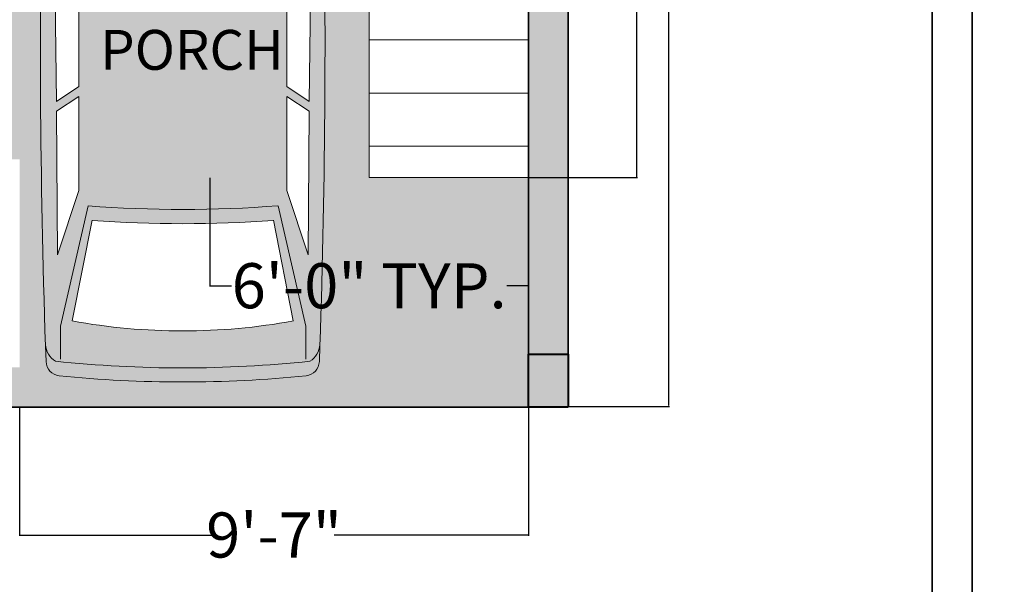
# Model space of a CAD drawing. Units: inches. Extents: x 1077 to 2505, y 1892 to 2728.
# Tile 7 of 26: x 1433 to 1655, y 2048 to 2176. Entities that reach past the tile are written whole.
import ezdxf

# ---------------------------------------------------------------- set-up
doc = ezdxf.new("R2010")
doc.units = ezdxf.units.IN
doc.linetypes.add('ACAD_ISO02W100', pattern=[15, 12, -3])
doc.layers.get('Defpoints').update_dxf_attribs({"color": 220, "linetype": 'ACAD_ISO02W100'})
for name, color, linetype, lineweight in [('A-ANNO-DIMS', 2, 'Continuous', 18), ('A-ANNO-TTLB', 7, 'Continuous', 35), ('A-AREA-IDEN', 7, 'Continuous', 18), ('A-COLS', 7, 'Continuous', 40), ('A-FLOR-STRS', 7, 'Continuous', 18), ('A-FURNITURE', 251, 'Continuous', 5), ('A-SITE-VEHI', 8, 'Continuous', 13), ('A-WALL-PATT', 7, 'Continuous', 9), ('WALL', 7, 'Continuous', 35)]:
    doc.layers.add(name, color=color, linetype=linetype, lineweight=lineweight)
doc.layers.add('A-FLOR-PATT', color=254, linetype='Continuous', lineweight=9, true_color=0xd7ebd2)
doc.styles.get("Standard").update_dxf_attribs({"font": 'arial.ttf'})
doc.dimstyles.get("Standard").update_dxf_attribs({"dimtxt": 10.18, "dimasz": 0.18, "dimexe": 0.18, "dimexo": 0.0625, "dimgap": 0.09, "dimtad": 0, "dimtih": 1, "dimtoh": 1, "dimdec": 0, "dimzin": 0, "dimdsep": 46, "dimlunit": 3, "dimtxsty": 'Standard', "dimcen": 0.09, "dimadec": 0, "dimazin": 0, "dimtfac": 1, "dimtdec": 0, "dimtofl": 0, "dimtmove": 0, "dimatfit": 3, "dimfxl": 1, "dimtolj": 1, "dimtzin": 0, "dimarcsym": 0})

# ---------------------------------------------------------------- blocks, each defined once
blk = doc.blocks.new('CAR')
at = {"layer": 'A-FURNITURE'}
for p, q in [((2677.91, 1665.57), (2683.24, 1629.33)), ((2722.63, 1665.57), (2717.3, 1629.33)), ((2672.85, 1620.44), (2676.61, 1608)), ((2727.48, 1620.44), (2723.73, 1608)), ((2671.15, 1614.07), (2676.73, 1600.01)), ((2671.63, 1575.61), (2671.15, 1614.07)), ((2729.25, 1614.07), (2723.67, 1600.01)), ((2728.77, 1575.61), (2729.25, 1614.07)), ((2676.73, 1600.01), (2676.73, 1578.97)), ((2723.67, 1600.01), (2723.67, 1578.97)), ((2676.73, 1578.97), (2671.63, 1575.61)), ((2723.67, 1578.97), (2728.77, 1575.61)), ((2676.73, 1576.71), (2671.66, 1573.38)), ((2676.73, 1576.71), (2676.73, 1555.46)), ((2723.67, 1576.71), (2723.67, 1555.46)), ((2723.67, 1576.71), (2728.74, 1573.38)), ((2671.9, 1540.91), (2671.66, 1573.38)), ((2728.49, 1540.91), (2728.74, 1573.38)), ((2676.73, 1555.46), (2671.9, 1540.91)), ((2723.67, 1555.46), (2728.49, 1540.91)), ((2678.77, 1552.01), (2672.52, 1524.85)), ((2721.71, 1552.02), (2727.96, 1524.85)), ((2675.22, 1526.01), (2679.74, 1548.74)), ((2725.17, 1526.01), (2720.66, 1548.74)), ((2672.52, 1524.85), (2672.52, 1517.39)), ((2727.96, 1524.85), (2727.96, 1517.39))]:
    blk.add_line(p, q, dxfattribs=at)
for centre, radius, start, end in [((2699.3, 1552.83), 119.14, 76.3976, 102.667), ((2674, 1665.84), 3.34, 104.3452, 166.6607), ((2699.3, 1570.19), 99.28, 73.0347, 105.8141), ((2726.43, 1665.41), 3.34, 13.1156, 74.5941), ((2783.1, 1639.97), 115.47, 166.6607, 186.5655), ((2673.27, 1662.52), 3.34, 107.8179, 168.3942), ((2727.17, 1661.99), 3.34, 11.3249, 70.8826), ((2617.23, 1639.97), 115.47, 353.4345, 13.1156), ((4741.11, 1589.62), 2073.11, 178.89024, 182.01225), ((2700.17, 1579.09), 51.94, 60.0774, 119.9226), ((659.22, 1589.62), 2073.11, 357.98775, 1.10976), ((2675.91, 1621.37), 3.2, 121.1455, 196.7984), ((2724.42, 1621.37), 3.2, 343.2016, 58.8545), ((2679.67, 1608.92), 3.2, 196.7984, 283.6631), ((2700.17, 1519.83), 88.22, 77.0683, 102.9317), ((2720.66, 1608.92), 3.2, 256.3369, 343.2016), ((2700.16, 1829.45), 278.26, 265.5919, 274.4407), ((2700.17, 1827.63), 279.65, 265.7971, 274.2029), ((2700.17, 1663.47), 139.72, 259.6897, 280.3103), ((2674.03, 1521.04), 4.9, 184.3987, 237.5288), ((2726.3, 1521.04), 4.9, 302.4712, 355.6013), ((2672.62, 1516.95), 3.34, 182.1119, 263.4899), ((2700.17, 1791.26), 275.86, 264.0142, 275.9858), ((2727.71, 1516.95), 3.34, 276.5101, 357.8881), ((2700.17, 1790.18), 277.96, 264.2342, 275.7658)]:
    blk.add_arc(centre, radius, start, end, dxfattribs=at)
blk = doc.blocks.new('C1')
h = blk.add_hatch(color=256)
h.dxf.hatch_style = 1
h.paths.add_polyline_path([(1668.56, 2445.41), (1677.56, 2445.41), (1677.56, 2457.41), (1668.56, 2457.41)])
for p, q in [((1668.56, 2457.41), (1677.56, 2457.41)), ((1668.56, 2445.41), (1668.56, 2457.41)), ((1677.56, 2457.41), (1677.56, 2445.41)), ((1677.56, 2445.41), (1668.56, 2445.41))]:
    blk.add_line(p, q)
blk = doc.blocks.new('*D14')
at = {"layer": 'A-ANNO-DIMS', "color": 0, "lineweight": -2, "transparency": 16777216}
for p, q in [((1555.59, 2651.66), (1579.43, 2651.66)), ((1579.25, 2651.48), (1579.25, 2375.3)), ((1579.25, 2088.54), (1579.25, 2364.72)), ((1555.59, 2088.36), (1579.43, 2088.36))]:
    blk.add_line(p, q, dxfattribs=at)
at = {"layer": 'A-ANNO-DIMS', "color": 0, "transparency": 16777216}
for points in [[(1579.22, 2651.48), (1579.28, 2651.48), (1579.25, 2651.66)], [(1579.22, 2088.54), (1579.28, 2088.54), (1579.25, 2088.36)]]:
    blk.add_solid(points, dxfattribs=at)
at = {"layer": 'Defpoints', "color": 0, "transparency": 16777216}
for p in [(1555.53, 2651.66), (1555.53, 2088.36), (1579.25, 2088.36)]:
    blk.add_point(p, dxfattribs=at)
at = {"layer": 'A-ANNO-DIMS', "color": 0, "transparency": 16777216, "insert": (1579.25, 2370.01), "char_height": 10.18, "attachment_point": 5}
blk.add_mtext('\\A1;46\'-11"', dxfattribs=at)
blk = doc.blocks.new('STAIR-PLAN-RETURN')
for p, q in [((0, 163.08), (0, 127.08)), ((12, 163.08), (12, 127.08)), ((24, 163.08), (24, 127.08)), ((36, 163.08), (36, 0)), ((36, 163.08), (36, 127.08)), ((0, 127.08), (72, 127.08)), ((36, 115.08), (72, 115.08)), ((36, 103.08), (72, 103.08)), ((36, 91.08), (72, 91.08)), ((36, 79.08), (72, 79.08)), ((36, 67.08), (72, 67.08)), ((36, 55.08), (72, 55.08)), ((36, 43.08), (72, 43.08)), ((36, 31.08), (72, 31.08)), ((36, 19.08), (72, 19.08)), ((36, 7.08), (72, 7.08)), ((72, 0), (36, 0))]:
    blk.add_line(p, q)
blk = doc.blocks.new('SHEET-FRAME-RESIDENTIAL')
for points in [[(0, 830.04), (543.52, 830.04), (543.52, 0), (0, 0)], [(9, 821.04), (534.52, 821.04), (534.52, 9), (9, 9)]]:
    blk.add_lwpolyline(points, close=True)
blk = doc.blocks.new('*D44')
at = {"layer": 'A-ANNO-DIMS', "color": 0, "lineweight": -2, "transparency": 16777216}
for p, q in [((1547.59, 2303.16), (1572.17, 2303.16)), ((1571.99, 2302.98), (1571.99, 2226.98)), ((1571.99, 2140.26), (1571.99, 2216.26)), ((1547.59, 2140.08), (1572.17, 2140.08))]:
    blk.add_line(p, q, dxfattribs=at)
at = {"layer": 'A-ANNO-DIMS', "color": 0, "transparency": 16777216}
for points in [[(1571.96, 2302.98), (1572.02, 2302.98), (1571.99, 2303.16)], [(1571.96, 2140.26), (1572.02, 2140.26), (1571.99, 2140.08)]]:
    blk.add_solid(points, dxfattribs=at)
at = {"layer": 'Defpoints', "color": 0, "transparency": 16777216}
for p in [(1547.53, 2303.16), (1571.99, 2303.16), (1547.53, 2140.08)]:
    blk.add_point(p, dxfattribs=at)
at = {"layer": 'A-ANNO-DIMS', "color": 0, "transparency": 16777216, "insert": (1571.99, 2221.62), "char_height": 10.18, "attachment_point": 5}
blk.add_mtext('\\A1;RETURN STAIR 13\'-7" TYP.', dxfattribs=at)
blk = doc.blocks.new('*D45')
at = {"layer": 'A-ANNO-DIMS', "color": 0, "lineweight": -2, "transparency": 16777216}
for p, q in [((1475.53, 2140.02), (1475.53, 2115.44)), ((1547.53, 2140.02), (1547.53, 2115.44)), ((1475.71, 2115.62), (1480.38, 2115.62)), ((1547.35, 2115.62), (1542.67, 2115.62))]:
    blk.add_line(p, q, dxfattribs=at)
at = {"layer": 'A-ANNO-DIMS', "color": 0, "transparency": 16777216}
for points in [[(1475.71, 2115.65), (1475.71, 2115.59), (1475.53, 2115.62)], [(1547.35, 2115.65), (1547.35, 2115.59), (1547.53, 2115.62)]]:
    blk.add_solid(points, dxfattribs=at)
at = {"layer": 'Defpoints', "color": 0, "transparency": 16777216}
for p in [(1475.53, 2140.08), (1547.53, 2140.08), (1547.53, 2115.62)]:
    blk.add_point(p, dxfattribs=at)
at = {"layer": 'A-ANNO-DIMS', "color": 0, "transparency": 16777216, "insert": (1511.53, 2115.62), "char_height": 10.18, "attachment_point": 5}
blk.add_mtext('\\A1;6\'-0" TYP.', dxfattribs=at)
blk = doc.blocks.new('*D67')
at = {"layer": 'A-ANNO-DIMS', "color": 0, "lineweight": -2, "transparency": 16777216}
for p, q in [((1432.53, 2088.1), (1432.53, 2059.13)), ((1547.53, 2088.1), (1547.53, 2059.13)), ((1432.71, 2059.31), (1476.41, 2059.31)), ((1547.35, 2059.31), (1503.65, 2059.31))]:
    blk.add_line(p, q, dxfattribs=at)
at = {"layer": 'A-ANNO-DIMS', "color": 0, "transparency": 16777216}
for points in [[(1432.71, 2059.34), (1432.71, 2059.28), (1432.53, 2059.31)], [(1547.35, 2059.34), (1547.35, 2059.28), (1547.53, 2059.31)]]:
    blk.add_solid(points, dxfattribs=at)
at = {"layer": 'Defpoints', "color": 0, "transparency": 16777216}
for p in [(1432.53, 2088.16), (1547.53, 2088.16), (1547.53, 2059.31)]:
    blk.add_point(p, dxfattribs=at)
at = {"layer": 'A-ANNO-DIMS', "color": 0, "transparency": 16777216, "insert": (1490.03, 2059.31), "char_height": 10.18, "attachment_point": 5}
blk.add_mtext('\\A1;9\'-7"', dxfattribs=at)

msp = doc.modelspace()

# ---------------------------------------------------------------- hatches: boundary and pattern name
at = {"layer": 'A-FLOR-PATT', "transparency": 33554559}
h = msp.add_hatch(color=256, dxfattribs=at)
h.dxf.hatch_style = 1
h.paths.add_polyline_path([(1395.53, 2577.16), (1374.83, 2577.16), (1350.83, 2577.19), (1350.83, 2577.16), (1329.53, 2577.16), (1329.53, 2480.16), (1329.53, 2469.16), (1325.53, 2469.16), (1325.53, 2515.13), (1307.53, 2515.13), (1307.53, 2577.16), (1269.31, 2577.16), (1221.31, 2577.15), (1221.31, 2577.16), (1187.53, 2577.16), (1187.53, 2433.16), (1289.53, 2433.16), (1289.53, 2429.16), (1263.53, 2429.16), (1187.53, 2429.16), (1187.53, 2395.02), (1187.53, 2395.02), (1187.53, 2371.02), (1187.53, 2371.02), (1187.53, 2307.16), (1259.53, 2307.16), (1259.53, 2399.16), (1263.53, 2399.16), (1263.53, 2307.16), (1289.53, 2307.16), (1289.53, 2306.23), (1325.53, 2306.23), (1325.53, 2307.16), (1329.53, 2307.16), (1329.53, 2306.23), (1365.53, 2306.23), (1365.53, 2307.16), (1432.53, 2307.16), (1432.53, 2088.16), (1547.53, 2088.16), (1547.53, 2140.08), (1511.53, 2140.08), (1511.53, 2267.16), (1475.53, 2267.16), (1475.53, 2303.16), (1468.53, 2303.16), (1468.53, 2307.16), (1547.53, 2307.16), (1547.53, 2348.22), (1547.53, 2396.22), (1547.53, 2429.16), (1435.53, 2429.16), (1435.53, 2433.16), (1476.35, 2433.16), (1476.35, 2451.18), (1547.53, 2451.18), (1547.53, 2577.16), (1499.53, 2577.16), (1499.53, 2586.16), (1547.53, 2586.16), (1547.53, 2642.16), (1518.18, 2642.16), (1518.18, 2642.05), (1494.15, 2642.05), (1494.15, 2642.16), (1469.53, 2642.16), (1469.53, 2577.16), (1399.53, 2577.16), (1399.53, 2429.16), (1325.53, 2429.16), (1325.53, 2433.16), (1329.53, 2433.16), (1395.53, 2433.16), (1395.53, 2480.16), (1359.53, 2480.16), (1359.53, 2484.16), (1395.53, 2484.16)])
h.paths.add_polyline_path([(1357.65, 2482.07), (1355.65, 2482.07), (1355.65, 2481.07, 0.414214), (1356.65, 2480.07), (1344.65, 2480.07), (1344.65, 2477.06), (1343.27, 2477.06), (1343.27, 2480.07), (1330.65, 2480.07, -0.414214), (1329.65, 2481.07), (1329.65, 2484.07), (1331.65, 2484.07), (1331.65, 2510.07, -0.446908)], flags=16)
h.paths.add_polyline_path([(1305.09, 2559.18), (1288.89, 2559.18), (1288.89, 2575.38), (1305.09, 2575.38)], flags=16)
h.paths.add_polyline_path([(1304.19, 2560.08), (1289.79, 2560.08), (1289.79, 2574.48), (1304.19, 2574.48)], flags=0)
h.paths.add_polyline_path([(1287.99, 2500.68, -0.414214), (1287.09, 2499.78), (1265.14, 2499.78), (1224.09, 2499.78, -0.414214), (1223.19, 2500.68), (1223.19, 2557.16), (1223.19, 2571.74), (1223.19, 2575.38), (1287.99, 2575.38), (1287.99, 2571.74), (1287.09, 2571.74, -0.414214), (1287.99, 2570.84)], flags=16)
h.paths.add_polyline_path([(1292.98, 2569.05, -1), (1300.92, 2569.05, -1)], flags=0)
h.paths.add_polyline_path([(1293.32, 2569.05, -1), (1300.58, 2569.05, -1)], flags=0)
h.paths.add_polyline_path([(1322.8, 2462.21), (1322.8, 2431.71), (1323.05, 2430.71), (1323.05, 2431.71), (1321.8, 2431.71), (1321.8, 2462.19, 0.404641), (1292.3, 2431.71), (1292.05, 2430.71, -0.414214), (1291.55, 2430.21), (1291.05, 2430.21), (1291.05, 2429.71, -0.414214), (1290.55, 2429.21), (1289.55, 2429.21), (1289.55, 2434.21), (1290.55, 2434.21, -0.414214), (1291.05, 2433.71), (1291.05, 2433.21), (1291.55, 2433.21, -0.414214), (1292.05, 2432.71), (1292.3, 2431.71, -0.414214)], flags=16)
h.paths.add_polyline_path([(1287.82, 2548.28, 0.292232), (1279.17, 2536.8, 0.052719), (1223.93, 2548.28), (1223.28, 2548.28), (1223.28, 2557.16), (1223.93, 2557.16), (1245.42, 2557.16, -0.117785), (1245.77, 2557.93, -0.059418), (1254.87, 2567.02, -0.379859), (1257.28, 2566.88, -0.02509), (1261.41, 2563.32, -0.025935), (1265.65, 2567.02, -0.379859), (1268.06, 2566.88, -0.061767), (1277.52, 2557.43, -0.069393), (1277.82, 2557.16), (1287.82, 2557.16)], flags=0)
h.paths.add_polyline_path([(1263.47, 2548.28), (1260.56, 2548.28, -0.015371), (1258.01, 2546.13, -0.429576), (1255.37, 2546.06, -0.016036), (1252.69, 2548.28), (1223.28, 2548.28), (1223.28, 2554.42), (1246.78, 2554.42, 0.055344), (1255.37, 2546.06, 0.331768), (1257.52, 2545.74, 0.027343), (1262, 2549.64, 0.00919)], flags=0)
h.paths.add_polyline_path([(1295.56, 2568.34), (1296.87, 2569.09), (1296.87, 2570.6, 0.399698), (1295.39, 2569.05, 0.119004)], flags=0)
h.paths.add_polyline_path([(1295.21, 2569.05, -1), (1298.68, 2569.05, -1)], flags=0)
h.paths.add_polyline_path([(1296.95, 2568.96), (1297.03, 2569), (1297.03, 2569.09), (1296.99, 2569.11), (1296.91, 2568.98)], flags=0)
h.paths.add_polyline_path([(1402.28, 2462.19, -0.414214), (1432.78, 2431.69), (1433.03, 2432.69), (1432.78, 2431.69, 0.404641), (1403.28, 2462.17), (1403.28, 2431.69), (1402.03, 2431.69), (1402.03, 2430.69, -0.414214), (1401.53, 2430.19), (1401.03, 2430.19), (1401.03, 2429.69, -0.414214), (1400.53, 2429.19), (1399.53, 2429.19), (1399.53, 2434.19), (1400.53, 2434.19, -0.414214), (1401.03, 2433.69), (1401.03, 2433.19), (1401.53, 2433.19, -0.414214), (1402.03, 2432.69)], flags=16)
h.paths.add_polyline_path([(1470.16, 2535.21, -0.414214), (1471.06, 2536.11), (1527.54, 2536.11), (1542.12, 2536.11), (1545.76, 2536.11), (1545.76, 2471.31), (1542.12, 2471.31), (1542.12, 2472.21, -0.414214), (1541.22, 2471.31), (1471.06, 2471.31, -0.414214), (1470.16, 2472.21), (1470.16, 2494.16)], flags=16)
h.paths.add_polyline_path([(1483.07, 2536.11, 0.253465), (1480.11, 2526.15, 0.2538), (1470.15, 2523.19)], flags=16)
h.paths.add_polyline_path([(1223.19, 2512.69, 0.253465), (1233.14, 2509.74, 0.2538), (1236.1, 2499.77)], flags=16)
h.paths.add_polyline_path([(1469.77, 2578.72), (1469.77, 2581.72), (1471.77, 2581.72), (1471.77, 2607.72, -0.01951), (1473.77, 2607.68), (1473.77, 2579.72), (1473.77, 2578.72, -0.414214), (1472.77, 2577.72), (1470.77, 2577.72, -0.414214)], flags=16)
h.paths.add_polyline_path([(1382.46, 2398.13), (1395.04, 2398.13), (1395.04, 2399.74), (1382.46, 2399.74)], flags=16)
h.paths.add_polyline_path([(1379.94, 2397.18), (1379.94, 2389.82), (1380.5, 2389.82), (1380.5, 2396.05, -0.41429), (1381.06, 2396.61), (1396.47, 2396.61, -0.414213), (1397.03, 2396.05), (1397.03, 2389.82), (1397.59, 2389.82), (1397.59, 2397.18)], flags=16)
h.paths.add_polyline_path([(1263.37, 2428.14), (1263.37, 2426.14, -0.414214), (1262.37, 2425.14), (1261.37, 2425.14), (1233.41, 2425.14, 0.400854), (1259.37, 2401.04), (1259.37, 2401.14), (1261.37, 2401.14, -0.446908), (1233.37, 2427.14), (1259.37, 2427.14), (1259.37, 2429.14), (1262.37, 2429.14, -0.414214)], flags=16)
h.paths.add_polyline_path([(1404.79, 2398.13), (1417.37, 2398.13), (1417.37, 2399.74), (1404.79, 2399.74)], flags=16)
h.paths.add_polyline_path([(1402.27, 2397.18), (1404.79, 2398.13), (1417.37, 2398.13), (1419.92, 2397.18)], flags=16)
h.paths.add_polyline_path([(1432.26, 2383.16), (1432.26, 2370.59), (1433.87, 2370.59), (1433.87, 2383.16)], flags=16)
h.paths.add_polyline_path([(1431.3, 2385.69), (1423.84, 2385.69), (1423.84, 2385.13), (1430.18, 2385.13, -0.41429), (1430.74, 2384.57), (1430.74, 2369.16, -0.414237), (1430.18, 2368.6), (1423.84, 2368.6), (1423.84, 2368.03), (1431.3, 2368.03)], flags=16)
h.paths.add_polyline_path([(1417.37, 2351.16), (1417.37, 2349.54), (1418.9, 2349.54, 0.414236), (1419.92, 2350.56), (1419.92, 2352.11)], flags=16)
h.paths.add_polyline_path([(1395.04, 2351.16), (1395.04, 2349.54), (1396.58, 2349.54, 0.414235), (1397.59, 2350.56), (1397.59, 2352.11)], flags=16)
h.paths.add_polyline_path([(1366.7, 2370.05), (1365.09, 2370.05), (1365.09, 2368.52, 0.414235), (1366.11, 2367.5), (1367.66, 2367.5)], flags=16)
h.paths.add_polyline_path([(1419.36, 2359.47), (1419.36, 2353.24, -0.41419), (1418.8, 2352.68), (1403.39, 2352.68, -0.414137), (1402.83, 2353.24), (1402.83, 2359.47), (1397.03, 2359.47), (1397.03, 2353.24, -0.414189), (1396.47, 2352.68), (1381.06, 2352.68, -0.414137), (1380.5, 2353.24), (1380.5, 2359.47)], flags=16)
h.paths.add_polyline_path([(1222.29, 2559.18), (1206.09, 2559.18), (1206.09, 2575.38), (1222.29, 2575.38)], flags=16)
h.paths.add_polyline_path([(1221.39, 2560.08), (1206.99, 2560.08), (1206.99, 2574.48), (1221.39, 2574.48)], flags=0)
h.paths.add_polyline_path([(1482, 2577.72), (1482, 2580.73), (1483.38, 2580.73), (1483.38, 2577.72), (1484.77, 2577.72), (1484.77, 2574.72), (1483.38, 2574.72), (1483.38, 2577.72)], flags=16)
h.paths.add_polyline_path([(1266.37, 2415.53), (1266.37, 2414.14), (1263.37, 2414.14), (1263.37, 2415.53), (1260.36, 2415.53), (1260.36, 2416.91), (1263.37, 2416.91), (1263.37, 2415.53)], flags=16)
h.paths.add_polyline_path([(1210.26, 2569.05, -1), (1218.19, 2569.05, -1)], flags=0)
h.paths.add_polyline_path([(1210.6, 2569.05, -1), (1217.85, 2569.05, -1)], flags=0)
h.paths.add_polyline_path([(1212.84, 2568.34), (1214.15, 2569.09), (1214.15, 2570.6, 0.399698), (1212.67, 2569.05, 0.119004)], flags=0)
h.paths.add_polyline_path([(1212.49, 2569.05, -1), (1215.96, 2569.05, -1)], flags=0)
h.paths.add_polyline_path([(1214.23, 2568.96), (1214.3, 2568.91), (1214.3, 2569)], flags=0)
h.paths.add_polyline_path([(1507.18, 2480.12, 0.052719), (1518.66, 2535.36), (1518.66, 2536.01), (1527.54, 2536.01), (1527.54, 2535.36), (1527.54, 2513.88, -0.117785), (1528.31, 2513.53, -0.059418), (1537.4, 2504.43, -0.379859), (1537.26, 2502.01, -0.02509), (1533.7, 2497.89, -0.025935), (1537.4, 2493.64, -0.379859), (1537.26, 2491.23, -0.061767), (1527.8, 2481.77, -0.069393), (1527.54, 2481.47), (1527.54, 2471.47), (1518.66, 2471.47, 0.292232)], flags=0)
h.paths.add_polyline_path([(1516.43, 2503.92, -0.016036), (1518.66, 2506.6), (1518.66, 2536.01), (1524.8, 2536.01), (1524.8, 2512.51, 0.055344), (1516.43, 2503.92, 0.331768), (1516.12, 2501.77, 0.027343), (1520.01, 2497.29, 0.00919), (1518.66, 2495.82), (1518.66, 2498.73, -0.015371), (1516.5, 2501.28, -0.429576)], flags=0)
h.paths.add_polyline_path([(1499.63, 2625.5, -0.171636), (1502.82, 2631.01), (1502.82, 2633.37), (1498.68, 2633.37, -0.414214), (1497.7, 2634.36), (1497.7, 2640.66, -0.414214), (1498.68, 2641.64), (1514.82, 2641.64, -0.414214), (1515.81, 2640.66), (1515.81, 2634.36, -0.414214), (1514.82, 2633.37), (1510.69, 2633.37), (1510.69, 2631.01, -0.171636), (1513.88, 2625.5, -0.258205), (1509.31, 2614.47), (1504.19, 2614.47, -0.258205)], flags=16)
h.paths.add_polyline_path([(1501.2, 2625.5, -0.171636), (1504.39, 2631.01), (1509.12, 2631.01, -0.171636), (1512.3, 2625.5, -0.210384), (1509.35, 2616.02), (1504.16, 2616.02, -0.210384)], flags=0)
h.paths.add_polyline_path([(1529.56, 2537.01), (1529.56, 2553.21), (1545.76, 2553.21), (1545.76, 2537.01)], flags=16)
h.paths.add_polyline_path([(1530.46, 2537.91), (1530.46, 2552.31), (1544.86, 2552.31), (1544.86, 2537.91)], flags=0)
h.paths.add_polyline_path([(1535.45, 2545.07, -1), (1543.39, 2545.07, -1)], flags=0)
h.paths.add_polyline_path([(1535.8, 2545.07, -1), (1543.05, 2545.07, -1)], flags=0)
h.paths.add_polyline_path([(1529.56, 2470.41), (1545.76, 2470.41), (1545.76, 2454.21), (1529.56, 2454.21)], flags=16)
h.paths.add_polyline_path([(1541.16, 2544.99), (1540.98, 2544.99, -0.544606), (1538.71, 2543.68), (1538.62, 2543.53, 0.547962)], flags=0)
h.paths.add_polyline_path([(1530.46, 2469.51), (1544.86, 2469.51), (1544.86, 2455.11), (1530.46, 2455.11)], flags=0)
h.paths.add_polyline_path([(1539.47, 2545.14), (1539.42, 2545.22), (1539.38, 2545.14)], flags=0)
h.paths.add_polyline_path([(1543.39, 2462.34, -1), (1535.45, 2462.34, -1)], flags=0)
h.paths.add_polyline_path([(1543.05, 2462.34, -1), (1535.8, 2462.34, -1)], flags=0)
h.paths.add_polyline_path([(1541.16, 2462.27), (1540.98, 2462.27, -0.544606), (1538.71, 2460.96), (1538.62, 2460.8, 0.547962)], flags=0)
h.paths.add_polyline_path([(1539.47, 2462.42), (1539.42, 2462.5), (1539.38, 2462.42)], flags=0)
h.paths.add_polyline_path([(1435.32, 2335.25, -0.414214), (1465.82, 2304.75), (1466.07, 2305.75), (1465.82, 2304.75, 0.404641), (1436.32, 2335.23), (1436.32, 2304.75), (1435.07, 2304.75), (1435.07, 2303.75, -0.414214), (1434.57, 2303.25), (1434.07, 2303.25), (1434.07, 2302.75, -0.414214), (1433.57, 2302.25), (1432.57, 2302.25), (1432.57, 2307.25), (1433.57, 2307.25, -0.414214), (1434.07, 2306.75), (1434.07, 2306.25), (1434.57, 2306.25, -0.414214), (1435.07, 2305.75)], flags=16)
h.paths.add_polyline_path([(1532.13, 2635.71), (1535.43, 2635.71), (1535.43, 2635.89), (1532.13, 2635.89)], flags=16)
edge = h.paths.add_edge_path(flags=16)
edge.add_arc((1535.98, 2632.67), 0.183, 270, 360)
edge.add_line((1536.17, 2632.67), (1536.17, 2639.82))
edge.add_line((1536.17, 2639.82), (1538.29, 2639.82))
edge.add_line((1538.29, 2639.82), (1538.29, 2641.82))
edge.add_line((1538.29, 2641.82), (1533.25, 2641.82))
edge.add_line((1533.25, 2641.82), (1533.25, 2639.82))
edge.add_line((1533.25, 2639.82), (1534.87, 2639.82))
edge.add_line((1534.87, 2639.82), (1534.87, 2639))
edge.add_line((1534.87, 2639), (1533.7, 2639))
edge.add_line((1533.7, 2639), (1533.7, 2639.82))
edge.add_line((1533.7, 2639.82), (1533.25, 2639.82))
edge.add_line((1533.25, 2639.82), (1533.25, 2641.82))
edge.add_line((1533.25, 2641.82), (1538.29, 2641.82))
edge.add_line((1538.29, 2641.82), (1538.29, 2641.34))
edge.add_line((1538.29, 2641.34), (1540.64, 2641.58))
edge.add_line((1540.64, 2641.58), (1540.64, 2641.82))
edge.add_line((1540.64, 2641.82), (1541.5, 2641.82))
edge.add_line((1541.5, 2641.82), (1541.5, 2641.25))
edge.add_line((1541.5, 2641.25), (1541.31, 2639.79))
edge.add_ellipse((1541.09, 2638.95), major_axis=(-1.08, 0), ratio=0.790849, start_angle=180, end_angle=255.2976, ccw=False)
edge.add_line((1542.17, 2638.95), (1542.17, 2638.38))
edge.add_ellipse((1541.09, 2638.38), major_axis=(-1.08, 0), ratio=0.790849, start_angle=0, end_angle=180, ccw=False)
edge.add_line((1540, 2638.38), (1540.01, 2638.87))
edge.add_ellipse((1541.09, 2638.95), major_axis=(-1.08, 0), ratio=0.790849, start_angle=284.7024, end_angle=364.0401, ccw=False)
edge.add_line((1540.78, 2639.75), (1540.78, 2641.25))
edge.add_line((1540.78, 2641.25), (1540.64, 2641.25))
edge.add_line((1540.64, 2641.25), (1538.29, 2641.01))
edge.add_line((1538.29, 2641.01), (1538.29, 2639.82))
edge.add_line((1538.29, 2639.82), (1536.17, 2639.82))
edge.add_line((1536.17, 2639.82), (1536.17, 2632.48))
edge.add_line((1536.17, 2632.48), (1535.98, 2632.48))
h.paths.add_polyline_path([(1496.32, 2250.34, -0.292371), (1498.9, 2247.83, -0.085148), (1501.21, 2208.85, -0.01331), (1500.27, 2098.5, -0.379287), (1497.22, 2095.28, -0.0502), (1441.54, 2095.28, -0.379287), (1438.5, 2098.5, -0.01331), (1437.56, 2208.85, -0.086132), (1439.96, 2248.26, -0.295116), (1442.59, 2250.78, -0.114238)], flags=16)
h.paths.add_polyline_path([(1495.16, 2205.84, -0.355389), (1496.7, 2202.1), (1492.94, 2189.65, -0.398275), (1489.12, 2187.47, 0.113332), (1449.64, 2187.47, -0.398275), (1445.82, 2189.65), (1442.06, 2202.1, -0.355394), (1443.6, 2205.84, -0.265725)], flags=0)
h.paths.add_polyline_path([(1440.37, 2195.72), (1445.94, 2181.67), (1445.94, 2160.63), (1440.84, 2157.26)], flags=0)
h.paths.add_polyline_path([(1498.46, 2195.72), (1497.99, 2157.26), (1492.88, 2160.63), (1492.88, 2181.67)], flags=0)
h.paths.add_polyline_path([(1445.94, 2158.37), (1445.94, 2137.12), (1441.12, 2122.56), (1440.87, 2155.03)], flags=0)
h.paths.add_polyline_path([(1492.88, 2158.37), (1497.96, 2155.03), (1497.71, 2122.56), (1492.88, 2137.12)], flags=0)
h.paths.add_polyline_path([(1489.88, 2130.4), (1494.39, 2107.67, -0.090102), (1444.44, 2107.65), (1448.95, 2130.39, 0.036636)], flags=0)
h.paths.add_polyline_path([(1447.54, 2159.34), (1497.44, 2159.34), (1497.44, 2177.89), (1447.54, 2177.89)], flags=8)
h.paths.add_polyline_path([(1196.44, 2354.84), (1246.65, 2354.84), (1246.65, 2388.43), (1196.44, 2388.43)], flags=24)
h.paths.add_polyline_path([(1296.09, 2360.25), (1353.81, 2360.25), (1353.81, 2393.84), (1296.09, 2393.84)], flags=24)
h.paths.add_polyline_path([(1400.72, 2471.85), (1470.63, 2471.85), (1470.63, 2505.44), (1400.72, 2505.44)], flags=24)
h.paths.add_polyline_path([(1324.78, 2448.48), (1394.95, 2448.48), (1394.95, 2467.02), (1324.78, 2467.02)], flags=24)
h.paths.add_polyline_path([(1335.08, 2531.43), (1389.67, 2531.43), (1389.67, 2565.02), (1335.08, 2565.02)], flags=24)
h.paths.add_polyline_path([(1225.76, 2460), (1295.67, 2460), (1295.67, 2493.58), (1225.76, 2493.58)], flags=24)
h = msp.add_hatch(color=256, dxfattribs=at)
h.dxf.hatch_style = 1
h.paths.add_polyline_path([(1547.53, 2348.22), (1547.53, 2396.22), (1547.53, 2425.11), (1547.53, 2425.11), (1547.53, 2429.16), (1435.53, 2429.16), (1434.03, 2429.21), (1434.03, 2430.19), (1433.03, 2430.19), (1432.78, 2431.69, 0.404641), (1403.28, 2462.17), (1403.28, 2431.69), (1402.03, 2431.69), (1402.03, 2430.19), (1401.03, 2430.19), (1401.03, 2429.19), (1399.53, 2429.19), (1399.53, 2429.19), (1399.53, 2429.16), (1334.67, 2429.16), (1334.67, 2423.95), (1325.67, 2423.95), (1325.67, 2429.16), (1325.53, 2429.16), (1324.05, 2429.24), (1324.05, 2430.21), (1323.05, 2430.21), (1323.05, 2431.71), (1321.8, 2431.71), (1321.8, 2462.19, 0.416544), (1292.05, 2430.73, -0.423614), (1291.55, 2430.21), (1291.05, 2430.21), (1291.05, 2429.21), (1289.55, 2429.21), (1289.53, 2429.21), (1289.53, 2429.16), (1263.37, 2429.16), (1263.37, 2415.53), (1266.37, 2415.53), (1266.37, 2414.14), (1263.37, 2414.14), (1263.37, 2399.16), (1263.53, 2399.16), (1263.53, 2307.16), (1289.53, 2307.16), (1289.53, 2306.23), (1323.26, 2306.23), (1323.26, 2307.21), (1332.26, 2307.21), (1365.53, 2306.23), (1365.53, 2307.16), (1432.53, 2307.16), (1432.57, 2307.16), (1432.57, 2307.25), (1434.07, 2307.25), (1434.07, 2306.25), (1435.32, 2306.25), (1435.32, 2335.25, -0.407346), (1466.07, 2305.73, -0.423614), (1466.57, 2306.25), (1467.07, 2306.25), (1467.07, 2307.25), (1468.57, 2307.25), (1547.53, 2307.16), (1547.53, 2307.2)])
h.paths.add_polyline_path([(1430.74, 2369.16), (1430.74, 2384.57, 0.41429), (1430.18, 2385.13), (1423.84, 2385.13), (1423.84, 2368.6), (1430.18, 2368.6, 0.414237)], flags=16)
h.paths.add_polyline_path([(1432.26, 2383.16), (1432.26, 2370.59), (1433.87, 2370.59), (1433.87, 2383.16)], flags=16)
h.paths.add_polyline_path([(1431.3, 2368.03), (1431.3, 2385.69), (1432.26, 2383.16), (1432.26, 2370.59)], flags=16)
h.paths.add_polyline_path([(1417.37, 2351.16), (1417.37, 2349.54), (1418.9, 2349.54, 0.414236), (1419.92, 2350.56), (1419.92, 2352.11)], flags=16)
h.paths.add_polyline_path([(1403.39, 2352.68), (1418.78, 2352.68, 0.42427), (1419.36, 2353.24), (1419.36, 2359.47), (1402.83, 2359.47), (1402.83, 2353.24, 0.414137)], flags=16)
h.paths.add_polyline_path([(1366.7, 2370.05), (1365.09, 2370.05), (1365.09, 2368.52, 0.414235), (1366.11, 2367.5), (1367.66, 2367.5)], flags=16)
h.paths.add_polyline_path([(1382.46, 2398.13), (1395.04, 2398.13), (1395.04, 2399.74), (1382.46, 2399.74)], flags=16)
h.paths.add_polyline_path([(1396.47, 2396.61), (1381.06, 2396.61, 0.41429), (1380.5, 2396.05), (1380.5, 2389.82), (1397.03, 2389.82), (1397.03, 2396.05, 0.414213)], flags=16)
h.paths.add_polyline_path([(1402.27, 2397.18), (1402.83, 2396.05, -0.414213), (1403.39, 2396.61)], flags=16)
h.paths.add_polyline_path([(1418.8, 2396.61), (1419.36, 2396.61), (1419.36, 2396.05, 0.414237)], flags=16)
h.paths.add_polyline_path([(1404.79, 2398.13), (1417.37, 2398.13), (1417.37, 2399.74), (1404.79, 2399.74)], flags=16)
h.paths.add_polyline_path([(1381.06, 2352.68, -0.414213), (1380.5, 2353.24), (1380.27, 2352.11)], flags=16)
h.paths.add_polyline_path([(1396.58, 2349.54), (1396.58, 2349.54), (1395.04, 2349.54), (1395.04, 2349.54), (1382.46, 2349.54), (1382.46, 2351.16), (1395.04, 2351.16), (1397.59, 2352.11), (1397.59, 2350.56, -0.414235)], flags=16)
h.paths.add_polyline_path([(1379.94, 2397.18), (1382.46, 2398.13), (1395.04, 2398.13), (1397.59, 2397.18)], flags=16)
h.paths.add_polyline_path([(1368.78, 2384.59, 0.414213), (1368.22, 2384.03), (1367.66, 2367.5), (1367.66, 2385.15)], flags=16)
h.paths.add_polyline_path([(1547.53, 2574.38), (1547.51, 2574.38), (1547.51, 2577.16), (1499.53, 2577.16), (1484.77, 2577.44), (1484.77, 2574.72), (1483.38, 2574.72), (1483.38, 2577.72), (1482, 2577.72), (1469.53, 2577.72), (1469.53, 2577.16), (1401.95, 2577.16), (1401.95, 2574.12), (1399.53, 2574.12), (1399.53, 2434.19), (1401.03, 2434.19), (1401.03, 2433.19), (1402.28, 2433.19), (1402.28, 2462.19, -0.407346), (1433.03, 2432.67, -0.423614), (1433.53, 2433.19), (1434.03, 2433.19), (1434.03, 2434.19), (1435.53, 2434.19), (1476.35, 2433.81), (1476.35, 2451.18), (1547.53, 2451.18)])
h.paths.add_polyline_path([(1470.16, 2535.21, -0.414214), (1471.06, 2536.11), (1527.54, 2536.11), (1542.12, 2536.11), (1545.76, 2536.11), (1545.76, 2471.31), (1542.12, 2471.31), (1542.12, 2472.21, -0.414214), (1541.22, 2471.31), (1471.06, 2471.31, -0.414214), (1470.16, 2472.21), (1470.16, 2494.16)], flags=16)
h.paths.add_polyline_path([(1483.07, 2536.11, 0.253465), (1480.11, 2526.15, 0.2538), (1470.15, 2523.19)], flags=16)
h.paths.add_polyline_path([(1525.55, 2481.52, -0.000893), (1524.8, 2482.24), (1524.8, 2471.47), (1527.54, 2471.47), (1527.54, 2472.12), (1527.54, 2481.47, -0.388819)], flags=0)
h.paths.add_polyline_path([(1518.66, 2536.01), (1527.54, 2536.01), (1527.54, 2535.36), (1527.54, 2513.88, -0.117785), (1528.31, 2513.53, -0.059418), (1537.4, 2504.43, -0.379859), (1537.26, 2502.01, -0.02509), (1533.7, 2497.89, 0.033431), (1528.3, 2502.74, 0.308459), (1526.25, 2502.88, 0.047827), (1518.66, 2495.82), (1518.66, 2498.73, -0.015371), (1516.5, 2501.28, -0.429576), (1516.43, 2503.92, -0.016036), (1518.66, 2506.6)], flags=0)
h.paths.add_polyline_path([(1529.56, 2537.01), (1529.56, 2553.21), (1545.76, 2553.21), (1545.76, 2537.01)], flags=16)
h.paths.add_polyline_path([(1530.46, 2537.91), (1530.46, 2552.31), (1544.86, 2552.31), (1544.86, 2537.91)], flags=0)
h.paths.add_polyline_path([(1535.8, 2545.07, -1), (1543.05, 2545.07, -1)], flags=0)
h.paths.add_polyline_path([(1541.16, 2544.99), (1540.98, 2544.99, -0.544606), (1538.71, 2543.68), (1538.62, 2543.53, 0.547962)], flags=0)
h.paths.add_polyline_path([(1539.47, 2545.14), (1539.42, 2545.22), (1539.38, 2545.14)], flags=0)
h.paths.add_polyline_path([(1529.56, 2470.41), (1545.76, 2470.41), (1545.76, 2454.21), (1529.56, 2454.21)], flags=16)
h.paths.add_polyline_path([(1530.46, 2469.51), (1544.86, 2469.51), (1544.86, 2455.11), (1530.46, 2455.11)], flags=0)
h.paths.add_polyline_path([(1535.8, 2462.34, -1), (1543.05, 2462.34, -1)], flags=0)
h.paths.add_polyline_path([(1541.16, 2462.27), (1540.98, 2462.27, -0.544606), (1538.71, 2460.96), (1538.62, 2460.8, 0.547962)], flags=0)
h.paths.add_polyline_path([(1539.47, 2462.42), (1539.42, 2462.5), (1539.38, 2462.42)], flags=0)
h.paths.add_polyline_path([(1395.53, 2574.12), (1392.95, 2574.12), (1392.95, 2577.16), (1374.83, 2577.16), (1350.83, 2577.19), (1350.83, 2577.16), (1332.07, 2577.16), (1332.07, 2574), (1329.53, 2574), (1329.53, 2484.07), (1331.65, 2484.07), (1331.65, 2510.07, -0.423677), (1357.76, 2484.07), (1359.53, 2484.07), (1359.53, 2484.16), (1395.53, 2484.16)], flags=17)
h.paths.add_polyline_path([(1395.53, 2480.16), (1359.06, 2480.16, 0.437533), (1359.53, 2481.55), (1359.53, 2484.16), (1395.53, 2484.16), (1395.53, 2574.12), (1392.95, 2574.12), (1392.95, 2577.16), (1374.83, 2577.16), (1350.83, 2577.19), (1350.83, 2577.16), (1332.07, 2577.16), (1332.07, 2574), (1329.53, 2574), (1329.53, 2484.07), (1329.65, 2484.07), (1329.65, 2481.07), (1329.53, 2480.16), (1329.53, 2469.16), (1325.53, 2469.16), (1325.53, 2515.13), (1307.53, 2515.13), (1307.53, 2577.16), (1269.31, 2577.16), (1221.31, 2577.15), (1221.31, 2577.16), (1187.61, 2577.16), (1187.61, 2574.03), (1187.53, 2433.16), (1289.55, 2433.16), (1289.55, 2434.21), (1291.05, 2434.21), (1291.05, 2433.21), (1292.05, 2433.21), (1292.3, 2431.71, -0.414214), (1322.8, 2462.21), (1323.05, 2432.71, -0.414214), (1323.55, 2433.21), (1324.05, 2433.21), (1324.05, 2434.21), (1325.67, 2434.21), (1325.67, 2435.95), (1334.67, 2435.95), (1334.67, 2433.16), (1395.53, 2433.16)])
h.paths.add_polyline_path([(1344.65, 2480.07), (1344.65, 2477.06), (1343.27, 2477.06), (1343.27, 2480.07), (1332.65, 2480.07, 0.414214), (1333.65, 2481.07), (1333.65, 2482.07), (1331.65, 2482.07), (1331.65, 2484.07), (1331.65, 2510.07, -0.446908), (1357.65, 2482.07), (1355.65, 2482.07), (1355.65, 2481.07, 0.414214), (1356.65, 2480.07)], flags=16)
h.paths.add_polyline_path([(1287.99, 2500.68, -0.414214), (1287.09, 2499.78), (1265.14, 2499.78), (1224.09, 2499.78, -0.414214), (1223.19, 2500.68), (1223.19, 2557.16), (1223.19, 2571.74), (1223.19, 2575.38), (1287.99, 2575.38), (1287.99, 2571.74), (1287.09, 2571.74, -0.414214), (1287.99, 2570.84)], flags=16)
h.paths.add_polyline_path([(1277.77, 2555.17, -0.000893), (1277.05, 2554.42), (1287.82, 2554.42), (1287.82, 2557.16), (1287.17, 2557.16), (1277.82, 2557.16, -0.388819)], flags=0)
h.paths.add_polyline_path([(1223.28, 2548.28), (1223.28, 2557.16), (1223.93, 2557.16), (1245.42, 2557.16, -0.117785), (1245.77, 2557.93, -0.059418), (1254.87, 2567.02, -0.379859), (1257.28, 2566.88, -0.02509), (1261.41, 2563.32, 0.033431), (1256.55, 2557.93, 0.308459), (1256.41, 2555.88, 0.047827), (1263.47, 2548.28), (1260.56, 2548.28, -0.015371), (1258.01, 2546.13, -0.429576), (1255.37, 2546.06, -0.016036), (1252.69, 2548.28)], flags=0)
h.paths.add_polyline_path([(1305.09, 2559.18), (1288.89, 2559.18), (1288.89, 2575.38), (1305.09, 2575.38)], flags=16)
h.paths.add_polyline_path([(1304.19, 2560.08), (1289.79, 2560.08), (1289.79, 2574.48), (1304.19, 2574.48)], flags=0)
h.paths.add_polyline_path([(1300.58, 2569.05, -1), (1293.32, 2569.05, -1)], flags=0)
h.paths.add_polyline_path([(1223.19, 2512.69, 0.253465), (1233.14, 2509.74, 0.2538), (1236.1, 2499.77)], flags=16)
h.paths.add_polyline_path([(1295.56, 2568.34), (1296.87, 2569.09), (1296.87, 2570.6, 0.399698), (1295.39, 2569.05, 0.119004)], flags=0)
h.paths.add_polyline_path([(1295.21, 2569.05, -1), (1298.68, 2569.05, -1)], flags=0)
h.paths.add_polyline_path([(1296.95, 2568.96), (1297.03, 2569), (1297.03, 2569.09), (1296.99, 2569.11), (1296.91, 2568.98)], flags=0)
h.paths.add_polyline_path([(1222.29, 2559.18), (1206.09, 2559.18), (1206.09, 2575.38), (1222.29, 2575.38)], flags=16)
h.paths.add_polyline_path([(1221.39, 2560.08), (1206.99, 2560.08), (1206.99, 2574.48), (1221.39, 2574.48)], flags=0)
h.paths.add_polyline_path([(1217.85, 2569.05, -1), (1210.6, 2569.05, -1)], flags=0)
h.paths.add_polyline_path([(1212.84, 2568.34), (1214.15, 2569.09), (1214.15, 2570.6, 0.399698), (1212.67, 2569.05, 0.119004)], flags=0)
h.paths.add_polyline_path([(1212.49, 2569.05, -1), (1215.96, 2569.05, -1)], flags=0)
h.paths.add_polyline_path([(1214.23, 2568.96), (1214.3, 2569), (1214.3, 2569.09), (1214.26, 2569.11), (1214.19, 2568.98)], flags=0)
h.paths.add_polyline_path([(1259.53, 2399.14), (1259.37, 2399.14), (1259.37, 2401.04, -0.423677), (1233.37, 2427.14), (1259.37, 2427.14), (1259.37, 2429.16), (1187.53, 2429.16), (1187.53, 2395.02), (1187.53, 2395.02), (1187.53, 2371.02), (1187.53, 2371.02), (1187.53, 2311.49), (1187.55, 2311.49), (1187.55, 2307.16), (1259.53, 2307.16)])
h.paths.add_polyline_path([(1323.26, 2295.21), (1323.26, 2304.23), (1289.53, 2304.23), (1289.53, 2303.16), (1187.55, 2303.16), (1187.55, 2299.49), (1178.53, 2299.49), (1178.53, 2267.66), (1178.53, 2219.66), (1182.03, 2219.66), (1182.03, 2267.67), (1184.03, 2267.67), (1184.03, 2219.66), (1187.53, 2219.66), (1187.53, 2153.16), (1228.13, 2153.16), (1276.13, 2153.16), (1276.13, 2153.16), (1324.54, 2153.16), (1324.54, 2154.67), (1325.54, 2154.67), (1325.54, 2155.92), (1296.54, 2155.92, -0.407346), (1326.06, 2186.67, -0.423614), (1325.54, 2187.17), (1325.54, 2187.67), (1324.54, 2187.67), (1324.54, 2189.17), (1325.43, 2295.21)])
h.paths.add_polyline_path([(1432.53, 2307.16), (1365.53, 2307.16), (1365.53, 2306.23), (1365.53, 2303.16), (1428.53, 2303.16), (1428.53, 2221.2), (1428.57, 2221.2), (1428.57, 2197.2), (1428.53, 2197.16), (1428.53, 2303.01), (1404.46, 2303.01), (1404.46, 2221.2), (1329.53, 2221.2), (1329.53, 2307.16), (1325.53, 2307.16), (1325.53, 2295.21), (1325.43, 2295.21), (1324.54, 2189.17), (1324.54, 2187.67), (1326.04, 2187.67, 1.016365), (1326.06, 2186.67, 0.407348), (1296.54, 2155.92), (1325.54, 2155.92), (1325.54, 2154.67), (1324.54, 2154.67), (1324.54, 2153.16), (1329.53, 2153.16), (1329.53, 2144.16), (1432.53, 2144.16)])
h.paths.add_polyline_path([(1361.95, 2194.26), (1361.95, 2193.16), (1329.53, 2193.16), (1329.53, 2189.16), (1329.54, 2188.17), (1329.54, 2189.16), (1329.53, 2189.16), (1329.53, 2193.16), (1361.95, 2193.16), (1361.95, 2196.26), (1409.95, 2196.26), (1409.95, 2194.26)], flags=16)
h.paths.add_polyline_path([(1377.02, 2200.5), (1345.91, 2200.5), (1345.91, 2218.4), (1347.87, 2218.4), (1347.87, 2219.18), (1374.75, 2219.18), (1374.75, 2218.4), (1377.02, 2218.4)], flags=16)
h.paths.add_polyline_path([(1367.07, 2210.7, -1), (1373.34, 2210.7, -1)], flags=0)
h.paths.add_polyline_path([(1349.92, 2210.7, -1), (1356.98, 2210.7, -1)], flags=0)
h.paths.add_polyline_path([(1405.95, 2256.57), (1405.95, 2277.6), (1427.86, 2277.6), (1427.86, 2256.57)], flags=16)
h.paths.add_polyline_path([(1412.92, 2258.68, -0.414201), (1410.93, 2260.67), (1410.93, 2273.62, -0.414239), (1412.92, 2275.61), (1423.88, 2275.61, -0.414227), (1425.87, 2273.62), (1425.87, 2260.67, -0.414214), (1423.88, 2258.68)], flags=0)
h.paths.add_polyline_path([(1407.61, 2263.66, -1), (1409.18, 2263.66, -1)], flags=0)
h.paths.add_polyline_path([(1407.61, 2267.14, -1), (1409.18, 2267.14, -1)], flags=0)
h.paths.add_polyline_path([(1416.91, 2267.15, -1), (1419.89, 2267.15, -1)], flags=0)
h.paths.add_polyline_path([(1407.61, 2270.63, -1), (1409.18, 2270.63, -1)], flags=0)
h.paths.add_polyline_path([(1475.53, 2303.16), (1468.57, 2303.16), (1468.57, 2302.25), (1467.07, 2302.25), (1467.07, 2303.25), (1466.07, 2303.25), (1465.82, 2304.75, 0.404641), (1436.32, 2335.23), (1436.32, 2304.75), (1435.07, 2304.75), (1435.07, 2303.25), (1434.07, 2303.25), (1434.07, 2302.25), (1432.53, 2302.25), (1432.53, 2144.16), (1432.53, 2088.16), (1547.52, 2088.16), (1547.52, 2100.19), (1547.52, 2140.08), (1511.53, 2140.08), (1511.53, 2267.16), (1475.53, 2267.16)])
h.paths.add_polyline_path([(1438.35, 2102.86, 0.033498), (1438.37, 2102.21, -0.000079)], flags=16)
h.paths.add_polyline_path([(1496.32, 2250.34, -0.292371), (1498.9, 2247.83, -0.085148), (1501.21, 2208.85, -0.012784), (1500.42, 2102.86, -0.033498), (1500.39, 2102.21, 0.012863), (1501.21, 2208.85, 0.077283), (1499.67, 2244.3, 0.265882), (1497.48, 2246.8, 0.14401), (1441.46, 2247.36, 0.270646), (1439.21, 2244.85, -0.007564), (1439.96, 2248.26, -0.295116), (1442.59, 2250.78, -0.114238)], flags=16)
h.paths.add_polyline_path([(1495.16, 2205.84, -0.355389), (1496.7, 2202.1), (1492.94, 2189.65, -0.398275), (1489.12, 2187.47, 0.113332), (1449.64, 2187.47, -0.398275), (1445.82, 2189.65), (1442.06, 2202.1, -0.355394), (1443.6, 2205.84, -0.265725)], flags=16)
h.paths.add_polyline_path([(1440.37, 2195.72), (1445.94, 2181.67), (1445.94, 2160.63), (1440.84, 2157.26)], flags=16)
h.paths.add_polyline_path([(1498.46, 2195.72), (1497.99, 2157.26), (1492.88, 2160.63), (1492.88, 2181.67)], flags=16)
h.paths.add_polyline_path([(1445.94, 2158.37), (1445.94, 2137.12), (1441.12, 2122.56), (1440.87, 2155.03)], flags=16)
h.paths.add_polyline_path([(1492.88, 2158.37), (1497.96, 2155.03), (1497.71, 2122.56), (1492.88, 2137.12)], flags=16)
h.paths.add_polyline_path([(1489.88, 2130.4), (1494.39, 2107.67, -0.090102), (1444.44, 2107.65), (1448.95, 2130.39, 0.036636)], flags=16)
h.paths.add_polyline_path([(1296.09, 2360.25), (1353.81, 2360.25), (1353.81, 2393.84), (1296.09, 2393.84)], flags=24)
h.paths.add_polyline_path([(1400.72, 2471.85), (1470.63, 2471.85), (1470.63, 2505.44), (1400.72, 2505.44)], flags=24)
h.paths.add_polyline_path([(1335.08, 2531.43), (1389.67, 2531.43), (1389.67, 2565.02), (1335.08, 2565.02)], flags=24)
h.paths.add_polyline_path([(1324.78, 2448.48), (1394.95, 2448.48), (1394.95, 2467.02), (1324.78, 2467.02)], flags=24)
h.paths.add_polyline_path([(1225.76, 2460), (1295.67, 2460), (1295.67, 2493.58), (1225.76, 2493.58)], flags=24)
h.paths.add_polyline_path([(1196.44, 2354.84), (1246.65, 2354.84), (1246.65, 2388.43), (1196.44, 2388.43)], flags=24)
h.paths.add_polyline_path([(1447.54, 2159.34), (1497.44, 2159.34), (1497.44, 2177.89), (1447.54, 2177.89)], flags=24)
at = {"layer": 'A-WALL-PATT', "transparency": 33554585}
h = msp.add_hatch(color=256, dxfattribs=at)
h.dxf.hatch_style = 1
h.paths.add_polyline_path([(1187.53, 2424), (1178.53, 2424), (1178.53, 2395.02), (1187.53, 2395.02)])
h.paths.add_polyline_path([(1187.53, 2371.02), (1178.53, 2371.02), (1178.53, 2311.49), (1187.53, 2311.49)])
h.paths.add_polyline_path([(1228.13, 2153.16), (1187.53, 2153.16), (1187.53, 2219.66), (1178.53, 2219.66), (1178.53, 2100.18), (1187.53, 2100.18), (1187.53, 2144.16), (1228.13, 2144.16)])
h.paths.add_polyline_path([(1432.53, 2097.16), (1187.53, 2097.16), (1187.53, 2100.18), (1178.53, 2100.18), (1178.53, 2088.16), (1432.53, 2088.16)])
h.paths.add_polyline_path([(1556.53, 2348.22), (1547.53, 2348.22), (1547.53, 2348.22), (1547.53, 2307.16), (1468.53, 2307.16), (1468.53, 2303.16), (1547.53, 2303.16), (1547.53, 2088.16), (1556.53, 2088.16)])
h.paths.add_polyline_path([(1556.53, 2425.11), (1547.53, 2425.11), (1547.53, 2396.22), (1556.53, 2396.22)])
h.paths.add_polyline_path([(1547.53, 2433.16), (1435.53, 2433.16), (1435.53, 2429.16), (1547.53, 2429.16)])
h.paths.add_polyline_path([(1556.53, 2574.38), (1547.53, 2574.38), (1547.53, 2451.18), (1547.55, 2451.18), (1547.55, 2437.11), (1556.53, 2437.11)])
h.paths.add_polyline_path([(1556.53, 2639.11), (1547.53, 2639.11), (1547.53, 2586.38), (1556.53, 2586.38)])
h.paths.add_polyline_path([(1556.53, 2639.11), (1547.53, 2639.11), (1547.53, 2642.16), (1518.18, 2642.16), (1518.18, 2642.05), (1494.18, 2642.05), (1494.18, 2651.05), (1518.15, 2651.05), (1518.15, 2651.16), (1556.53, 2651.16)])
h.paths.add_polyline_path([(1494.15, 2651.16), (1469.6, 2651.16), (1469.6, 2642.16), (1494.15, 2642.16)])
h.paths.add_polyline_path([(1221.31, 2577.16), (1187.61, 2577.16), (1187.61, 2574.03), (1178.61, 2574.03), (1178.61, 2586.16), (1221.31, 2586.16)])
h.paths.add_polyline_path([(1323.07, 2586.16), (1269.31, 2586.16), (1269.31, 2577.16), (1323.07, 2577.16)])
h.paths.add_polyline_path([(1374.84, 2586.19), (1374.84, 2577.19), (1350.84, 2577.19), (1350.83, 2577.19), (1350.83, 2577.16), (1332.07, 2577.16), (1332.07, 2574), (1323.07, 2574), (1323.07, 2586.16), (1350.83, 2586.16), (1350.84, 2586.16), (1350.84, 2586.19)])
h.paths.add_polyline_path([(1392.95, 2586.16), (1374.84, 2586.16), (1374.84, 2577.16), (1392.95, 2577.16)], flags=17)
h.paths.add_polyline_path([(1469.53, 2642.16), (1469.6, 2651.16), (1460.53, 2651.16), (1460.53, 2586.16), (1392.95, 2586.16), (1392.95, 2577.16), (1395.53, 2577.16), (1395.53, 2484.16), (1359.53, 2484.16), (1359.53, 2480.16), (1395.53, 2480.16), (1395.53, 2433.16), (1329.53, 2433.16), (1325.53, 2433.16), (1325.53, 2429.16), (1399.53, 2429.16), (1399.53, 2577.16), (1469.53, 2577.16)])
h.paths.add_polyline_path([(1187.53, 2574.03), (1178.53, 2574.03), (1178.53, 2436), (1187.53, 2436)])

# ---------------------------------------------------------------- linework, layer by layer
at = {"layer": 'WALL'}
for p, q in [((1556.53, 2348.22), (1556.53, 2088.16)), ((1547.53, 2303.16), (1547.53, 2088.16)), ((1556.53, 2088.16), (1178.53, 2088.16))]:
    msp.add_line(p, q, dxfattribs=at)

# ---------------------------------------------------------------- block references
at = {"layer": 'A-ANNO-TTLB'}
msp.add_blockref('SHEET-FRAME-RESIDENTIAL', (1104.25, 1892.27), dxfattribs=at)
at = {"layer": 'A-COLS'}
msp.add_blockref('C1', (-121.04, -357.22), dxfattribs=at)
at = {"layer": 'A-FLOR-STRS'}
msp.add_blockref('STAIR-PLAN-RETURN', (1475.53, 2140.08), dxfattribs=at)
at = {"layer": 'A-SITE-VEHI'}
msp.add_blockref('CAR', (-1230.78, 581.66), dxfattribs=at)

# ---------------------------------------------------------------- texts
at = {"layer": 'A-AREA-IDEN', "insert": (1450.76, 2173.41), "char_height": 9, "attachment_point": 1}
msp.add_mtext_dynamic_manual_height_columns('PORCH', width=128.1076, gutter_width=12.5, heights=[0], dxfattribs=at)

# ---------------------------------------------------------------- dimensions: what is measured, and where the dimension line sits
at = {"layer": 'A-ANNO-DIMS'}
dim = msp.add_linear_dim(base=(1579.25, 2088.36), p1=(1555.53, 2651.66), p2=(1555.53, 2088.36), angle=90, dimstyle='Standard', override={"dimclrd": 0, "dimclre": 0, "dimclrt": 0}, dxfattribs=at)
dim.commit()
dim.dimension.update_dxf_attribs({"geometry": '*D14', "text_midpoint": (1579.25, 2370.01)})
dim = msp.add_linear_dim(base=(1571.99, 2303.16), p1=(1547.53, 2140.08), p2=(1547.53, 2303.16), angle=90, text='RETURN STAIR <> TYP.', dimstyle='Standard', override={"dimdec": 1, "dimlfac": 1, "dimrnd": 0, "dimzin": 1, "dimdsep": 46, "dimlunit": 4, "dimfrac": 2}, dxfattribs=at)
dim.commit()
dim.dimension.update_dxf_attribs({"geometry": '*D44', "text_midpoint": (1571.99, 2221.62)})
dim = msp.add_linear_dim(base=(1547.53, 2115.62), p1=(1475.53, 2140.08), p2=(1547.53, 2140.08), text='<> TYP.', dimstyle='Standard', override={"dimdec": 1, "dimlfac": 1, "dimrnd": 0, "dimzin": 1, "dimdsep": 46, "dimlunit": 4, "dimfrac": 2}, dxfattribs=at)
dim.commit()
dim.dimension.update_dxf_attribs({"geometry": '*D45', "text_midpoint": (1511.53, 2115.62)})
dim = msp.add_linear_dim(base=(1547.53, 2059.31), p1=(1432.53, 2088.16), p2=(1547.53, 2088.16), dimstyle='Standard', override={"dimdec": 1, "dimlfac": 1, "dimrnd": 0, "dimzin": 1, "dimdsep": 46, "dimlunit": 4, "dimfrac": 2}, dxfattribs=at)
dim.commit()
dim.dimension.update_dxf_attribs({"geometry": '*D67', "text_midpoint": (1490.03, 2059.31)})

doc.saveas('drawing.dxf')
